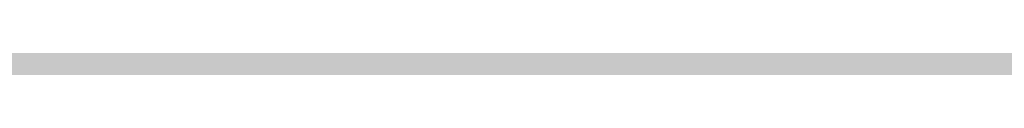
# Model space of a CAD drawing. Units: millimetres. Extents: x 0 to 2267, y 0 to 1823.
# Tile 79 of 256: x 1600.369 to 1605.705, y 1227.196 to 1227.23. Entities that reach past the tile are written whole.
import ezdxf

# ---------------------------------------------------------------- set-up
doc = ezdxf.new("R2010")
doc.units = ezdxf.units.MM
doc.header["$MEASUREMENT"] = 0
doc.layers.add('M-HATC', color=252, linetype='Continuous', lineweight=18)

msp = doc.modelspace()

# ---------------------------------------------------------------- hatches: boundary and pattern name
at = {"layer": 'M-HATC'}
h = msp.add_hatch(color=256, dxfattribs=at)
h.dxf.hatch_style = 1
h.paths.add_polyline_path([(2055.771, 1603.062), (1381.0868, 1603.062), (1381.0868, 1598.062), (2055.771, 1598.062)])
h.paths.add_polyline_path([(2055.771, 1598.062), (1381.0868, 1598.062), (1381.0868, 1593.062), (2055.771, 1593.062)])
h.paths.add_polyline_path([(2051.3074, 1536.7609), (1385.5504, 1536.7609), (1385.5504, 1526.7609), (1387.5504, 1526.7609), (1388.5366, 1525.0528), (1385.3319, 1521.2335), (1385.3319, 1521.2226), (2050.2542, 1522.7491), (2048.3212, 1525.0528), (2049.3074, 1526.7609), (2051.3074, 1526.7609)])
edge = h.paths.add_edge_path()
edge.add_arc((1847.5345, 1379.1492), 135, 222.603061, 222.890851, ccw=False)
edge.add_line((1748.1663, 1287.7656), (1683.0921, 1287.7656))
edge.add_arc((1583.7239, 1379.1492), 135, 317.109149, 317.396939, ccw=False)
edge.add_arc((1678.9686, 1290.6707), 5, 222.8909, 317.1091, ccw=False)
edge.add_arc((1774.2133, 1379.1492), 135, 222.603061, 222.890851, ccw=False)
edge.add_line((1674.8451, 1287.7656), (1609.7709, 1287.7656))
edge.add_arc((1510.4027, 1379.1492), 135, 317.109149, 317.396939, ccw=False)
edge.add_arc((1605.6474, 1290.6707), 5, 222.8909, 317.1091, ccw=False)
edge.add_arc((1700.8921, 1379.1492), 135, 222.603061, 222.890851, ccw=False)
edge.add_line((1601.5239, 1287.7656), (1536.4497, 1287.7656))
edge.add_arc((1437.0815, 1379.1492), 135, 317.109149, 317.396939, ccw=False)
edge.add_arc((1532.3262, 1290.6707), 5, 222.8909, 317.1091, ccw=False)
edge.add_arc((1627.5709, 1379.1492), 135, 222.603061, 222.890851, ccw=False)
edge.add_line((1528.2027, 1287.7656), (1505.9289, 1287.7656))
edge.add_spline(control_points=[(1505.9289, 1287.7656), (1504.2622, 1287.7656), (1504.2622, 1282.7656), (1505.9289, 1282.7656)], knot_values=[0, 0, 0, 0, 5, 5, 5, 5], degree=3, periodic=0)
edge.add_line((1505.9289, 1282.7656), (1930.9289, 1282.7656))
edge.add_spline(control_points=[(1930.9289, 1282.7656), (1932.5956, 1282.7656), (1932.5956, 1287.7656), (1930.9289, 1287.7656)], knot_values=[0, 0, 0, 0, 5, 5, 5, 5], degree=3, periodic=0)
edge.add_line((1930.9289, 1287.7656), (1903.0557, 1287.7656))
edge.add_arc((1803.6875, 1379.1492), 135, 317.109149, 317.396939, ccw=False)
edge.add_arc((1898.9322, 1290.6707), 5, 222.8909, 317.1091, ccw=False)
edge.add_arc((1994.1769, 1379.1492), 135, 222.603061, 222.890851, ccw=False)
edge.add_line((1894.8087, 1287.7656), (1829.7345, 1287.7656))
edge.add_arc((1730.3663, 1379.1492), 135, 317.109149, 317.396939, ccw=False)
edge.add_arc((1825.611, 1290.6707), 5, 222.8909, 317.1091, ccw=False)
edge.add_arc((1920.8557, 1379.1492), 135, 222.603061, 222.890851, ccw=False)
edge.add_line((1821.4875, 1287.7656), (1756.4133, 1287.7656))
edge.add_arc((1657.0451, 1379.1492), 135, 317.109149, 317.396939, ccw=False)
edge.add_arc((1752.2898, 1290.6707), 5, 222.8909, 317.1091, ccw=False)
edge = h.paths.add_edge_path()
edge.add_spline(control_points=[(1843.4289, 1227.2475), (1845.0956, 1227.2475), (1845.0956, 1232.2475), (1843.4289, 1232.2475)], knot_values=[0, 0, 0, 0, 5, 5, 5, 5], degree=3, periodic=0)
edge.add_line((1843.4289, 1232.2475), (1593.4289, 1232.2475))
edge.add_spline(control_points=[(1593.4289, 1232.2475), (1591.7622, 1232.2475), (1591.7622, 1227.2475), (1593.4289, 1227.2475)], knot_values=[0, 0, 0, 0, 5, 5, 5, 5], degree=3, periodic=0)
edge.add_line((1593.4289, 1227.2475), (1843.4289, 1227.2475))
h.paths.add_polyline_path([(1905.9289, 1127.4171), (1530.9289, 1127.4171, 0.414214), (1520.9289, 1117.4171), (1530.9289, 1117.4171), (1915.9289, 1117.4171, 0.414214)])
edge = h.paths.add_edge_path()
edge.add_arc((1397.0858, 1498.4078), 12.7299, 90.78215, 190.87871, ccw=False)
edge.add_line((1396.912, 1511.1365), (1428.0097, 1511.3488))
edge.add_line((1428.0097, 1511.3488), (1433.0097, 1511.3488))
edge.add_line((1433.0097, 1511.3488), (1434.439, 1511.3488))
edge.add_arc((1419.474, 1498.0804), 20, 41.561, 74.08211)
edge.add_line((1424.9592, 1517.3135), (1399.9351, 1517.2561))
edge.add_spline(control_points=[(1399.9307, 1517.2561), (1399.884, 1517.2131), (1399.8328, 1517.1689), (1399.7774, 1517.1236)], knot_values=[11.567499, 11.567499, 11.567499, 11.567499, 11.814249, 11.814249, 11.814249, 11.814249], degree=3, periodic=0)
edge.add_spline(control_points=[(1399.6328, 1517.0099), (1399.5831, 1516.9721), (1399.5307, 1516.9338), (1399.4759, 1516.8947)], knot_values=[11.167718, 11.167718, 11.167718, 11.167718, 11.365188, 11.365188, 11.365188, 11.365188], degree=3, periodic=0)
edge.add_spline(control_points=[(1399.3398, 1516.8001), (1399.1514, 1516.6719), (1398.9384, 1516.5377), (1398.704, 1516.3994)], knot_values=[10.376405, 10.376405, 10.376405, 10.376405, 11.00994, 11.00994, 11.00994, 11.00994], degree=3, periodic=0)
edge.add_spline(control_points=[(1398.6572, 1516.3719), (1398.5789, 1516.326), (1398.4983, 1516.2797), (1398.4155, 1516.2331)], knot_values=[10.125175, 10.125175, 10.125175, 10.125175, 10.334406, 10.334406, 10.334406, 10.334406], degree=3, periodic=0)
edge.add_spline(control_points=[(1398.2642, 1516.1487), (1398.196, 1516.1111), (1398.1263, 1516.0732), (1398.0555, 1516.0351)], knot_values=[9.832246, 9.832246, 9.832246, 9.832246, 9.999658, 9.999658, 9.999658, 9.999658], degree=3, periodic=0)
edge.add_spline(control_points=[(1397.9987, 1516.0048), (1397.7312, 1515.8621), (1397.446, 1515.7171), (1397.1466, 1515.5714)], knot_values=[9.161808, 9.161808, 9.161808, 9.161808, 9.787769, 9.787769, 9.787769, 9.787769], degree=3, periodic=0)
edge.add_spline(control_points=[(1397.1466, 1515.5714), (1396.8418, 1515.423), (1396.5222, 1515.274), (1396.1914, 1515.1262)], knot_values=[8.524455, 8.524455, 8.524455, 8.524455, 9.161808, 9.161808, 9.161808, 9.161808], degree=3, periodic=0)
edge.add_spline(control_points=[(1396.0777, 1515.0756), (1395.9854, 1515.0348), (1395.8922, 1514.994), (1395.7983, 1514.9534)], knot_values=[8.275193, 8.275193, 8.275193, 8.275193, 8.451726, 8.451726, 8.451726, 8.451726], degree=3, periodic=0)
edge.add_spline(control_points=[(1395.6018, 1514.8691), (1395.4997, 1514.8257), (1395.3968, 1514.7824), (1395.2932, 1514.7394)], knot_values=[7.962917, 7.962917, 7.962917, 7.962917, 8.152764, 8.152764, 8.152764, 8.152764], degree=3, periodic=0)
edge.add_spline(control_points=[(1395.2116, 1514.7057), (1394.8278, 1514.5475), (1394.4345, 1514.3929), (1394.0364, 1514.2442)], knot_values=[7.21254, 7.21254, 7.21254, 7.21254, 7.913148, 7.913148, 7.913148, 7.913148], degree=3, periodic=0)
edge.add_spline(control_points=[(1394.0364, 1514.2442), (1393.7076, 1514.1214), (1393.3754, 1514.0027), (1393.0427, 1513.8895)], knot_values=[6.633733, 6.633733, 6.633733, 6.633733, 7.21254, 7.21254, 7.21254, 7.21254], degree=3, periodic=0)
edge.add_spline(control_points=[(1392.8214, 1513.815), (1392.7198, 1513.7812), (1392.6181, 1513.7479), (1392.5166, 1513.7152)], knot_values=[6.328796, 6.328796, 6.328796, 6.328796, 6.505493, 6.505493, 6.505493, 6.505493], degree=3, periodic=0)
edge.add_spline(control_points=[(1392.5166, 1513.7152), (1392.3187, 1513.6515), (1392.1212, 1513.59), (1391.9244, 1513.531)], knot_values=[5.984605, 5.984605, 5.984605, 5.984605, 6.328796, 6.328796, 6.328796, 6.328796], degree=3, periodic=0)
edge.add_spline(control_points=[(1391.7915, 1513.4915), (1391.3122, 1513.3501), (1390.8384, 1513.2239), (1390.3784, 1513.1171)], knot_values=[5.066697, 5.066697, 5.066697, 5.066697, 5.907055, 5.907055, 5.907055, 5.907055], degree=3, periodic=0)
edge.add_spline(control_points=[(1390.3784, 1513.1171), (1390.1797, 1513.071), (1389.9836, 1513.0284), (1389.7907, 1512.9899)], knot_values=[4.70367, 4.70367, 4.70367, 4.70367, 5.066695, 5.066695, 5.066695, 5.066695], degree=3, periodic=0)
edge.add_spline(control_points=[(1389.422, 1512.9204), (1389.2459, 1512.8892), (1389.0729, 1512.8617), (1388.9036, 1512.8381)], knot_values=[4.130571, 4.130571, 4.130571, 4.130571, 4.469816, 4.469816, 4.469816, 4.469816], degree=3, periodic=0)
edge.add_spline(control_points=[(1388.9036, 1512.8381), (1388.591, 1512.7946), (1388.2911, 1512.7644), (1388.0071, 1512.7494)], knot_values=[3.504031, 3.504031, 3.504031, 3.504031, 4.130571, 4.130571, 4.130571, 4.130571], degree=3, periodic=0)
edge.add_spline(control_points=[(1387.9356, 1512.7459), (1387.8538, 1512.7423), (1387.7733, 1512.74), (1387.6944, 1512.739)], knot_values=[3.268866, 3.268866, 3.268866, 3.268866, 3.451164, 3.451164, 3.451164, 3.451164], degree=3, periodic=0)
edge.add_spline(control_points=[(1387.3351, 1512.7443), (1387.2076, 1512.7499), (1387.0847, 1512.7597), (1386.967, 1512.7739)], knot_values=[2.670686, 2.670686, 2.670686, 2.670686, 2.984, 2.984, 2.984, 2.984], degree=3, periodic=0)
edge.add_spline(control_points=[(1386.8327, 1512.7922), (1386.8209, 1512.7941), (1386.8092, 1512.7959), (1386.7975, 1512.7979)], knot_values=[2.516981, 2.516981, 2.516981, 2.516981, 2.549528, 2.549528, 2.549528, 2.549528], degree=3, periodic=0)
edge.add_spline(control_points=[(1386.4526, 1512.8735), (1386.4257, 1512.881), (1386.3993, 1512.889), (1386.3733, 1512.8972)], knot_values=[2.095869, 2.095869, 2.095869, 2.095869, 2.17941, 2.17941, 2.17941, 2.17941], degree=3, periodic=0)
edge.add_spline(control_points=[(1386.0691, 1513.0189), (1386.0634, 1513.0217), (1386.0577, 1513.0246), (1386.052, 1513.0275)], knot_values=[1.72453, 1.72453, 1.72453, 1.72453, 1.745933, 1.745933, 1.745933, 1.745933], degree=3, periodic=0)
edge.add_arc((1399.474, 1498.0804), 20, 131.82432, 180)
edge.add_arc((1630.3336, 1505.5484), 250.9708, 181.705176, 236.427975)
edge.add_arc((1605.3399, 1483.3044), 218.7822, 238.660829, 243.34961)
edge.add_arc((1647.0911, 1510.3592), 262.8986, 183.129836, 237.853442, ccw=False)
h.paths.add_polyline_path([(1406.5369, 1391.9644, 0.149382), (1491.5506, 1296.4418, -0.129517)], flags=17)
edge = h.paths.add_edge_path()
edge.add_arc((2037.3838, 1498.0804), 20, 0, 48.26587)
edge.add_spline(control_points=[(2050.6973, 1513.0052), (2050.6512, 1512.9847), (2050.6034, 1512.9655), (2050.5539, 1512.9477)], knot_values=[1.835652, 1.835652, 1.835652, 1.835652, 2.000781, 2.000781, 2.000781, 2.000781], degree=3, periodic=0)
edge.add_spline(control_points=[(2050.4616, 1512.9166), (2050.479, 1512.9221), (2050.4963, 1512.9277), (2050.5133, 1512.9335)], knot_values=[2.045477, 2.045477, 2.045477, 2.045477, 2.101389, 2.101389, 2.101389, 2.101389], degree=3, periodic=0)
edge.add_spline(control_points=[(2050.129, 1512.8342), (2050.1984, 1512.8473), (2050.2657, 1512.8623), (2050.3308, 1512.8792)], knot_values=[2.237629, 2.237629, 2.237629, 2.237629, 2.435841, 2.435841, 2.435841, 2.435841], degree=3, periodic=0)
edge.add_spline(control_points=[(2050.0946, 1512.8278), (2050.1061, 1512.8299), (2050.1176, 1512.832), (2050.129, 1512.8342)], knot_values=[2.435841, 2.435841, 2.435841, 2.435841, 2.468321, 2.468321, 2.468321, 2.468321], degree=3, periodic=0)
edge.add_spline(control_points=[(2049.7843, 1512.7851), (2049.8552, 1512.7922), (2049.9243, 1512.8008), (2049.9917, 1512.8109)], knot_values=[2.563852, 2.563852, 2.563852, 2.563852, 2.748541, 2.748541, 2.748541, 2.748541], degree=3, periodic=0)
edge.add_spline(control_points=[(2049.4052, 1512.7617), (2049.5364, 1512.7653), (2049.6629, 1512.773), (2049.7843, 1512.7851)], knot_values=[2.748541, 2.748541, 2.748541, 2.748541, 3.064882, 3.064882, 3.064882, 3.064882], degree=3, periodic=0)
edge.add_spline(control_points=[(2049.1698, 1512.7597), (2049.2336, 1512.7591), (2049.2965, 1512.7594), (2049.3584, 1512.7606)], knot_values=[3.102309, 3.102309, 3.102309, 3.102309, 3.2503, 3.2503, 3.2503, 3.2503], degree=3, periodic=0)
edge.add_spline(control_points=[(2048.8573, 1512.7691), (2048.9638, 1512.7638), (2049.068, 1512.7606), (2049.1698, 1512.7597)], knot_values=[3.2503, 3.2503, 3.2503, 3.2503, 3.486069, 3.486069, 3.486069, 3.486069], degree=3, periodic=0)
edge.add_spline(control_points=[(2048.6924, 1512.7789), (2048.3729, 1512.8009), (2048.0345, 1512.8411), (2047.6817, 1512.897)], knot_values=[3.606429, 3.606429, 3.606429, 3.606429, 4.2989, 4.2989, 4.2989, 4.2989], degree=3, periodic=0)
edge.add_spline(control_points=[(2047.6817, 1512.897), (2047.5458, 1512.9185), (2047.4077, 1512.9424), (2047.2678, 1512.9685)], knot_values=[4.2989, 4.2989, 4.2989, 4.2989, 4.565769, 4.565769, 4.565769, 4.565769], degree=3, periodic=0)
edge.add_spline(control_points=[(2047.2678, 1512.9685), (2047.1449, 1512.9914), (2047.0207, 1513.016), (2046.8951, 1513.0422)], knot_values=[4.565769, 4.565769, 4.565769, 4.565769, 4.799971, 4.799971, 4.799971, 4.799971], degree=3, periodic=0)
edge.add_spline(control_points=[(2046.8951, 1513.0422), (2046.5286, 1513.1188), (2046.1513, 1513.209), (2045.7676, 1513.3107)], knot_values=[4.799971, 4.799971, 4.799971, 4.799971, 5.483718, 5.483718, 5.483718, 5.483718], degree=3, periodic=0)
edge.add_spline(control_points=[(2045.7676, 1513.3107), (2045.3724, 1513.4154), (2044.9704, 1513.5322), (2044.5662, 1513.6588)], knot_values=[5.483718, 5.483718, 5.483718, 5.483718, 6.187866, 6.187866, 6.187866, 6.187866], degree=3, periodic=0)
edge.add_spline(control_points=[(2044.5662, 1513.6588), (2044.4149, 1513.7061), (2044.2633, 1513.7549), (2044.1116, 1513.8048)], knot_values=[6.187866, 6.187866, 6.187866, 6.187866, 6.451551, 6.451551, 6.451551, 6.451551], degree=3, periodic=0)
edge.add_spline(control_points=[(2044.1116, 1513.8048), (2043.9967, 1513.8427), (2043.8817, 1513.8813), (2043.7668, 1513.9205)], knot_values=[6.451551, 6.451551, 6.451551, 6.451551, 6.651434, 6.651434, 6.651434, 6.651434], degree=3, periodic=0)
edge.add_spline(control_points=[(2043.7668, 1513.9205), (2043.3716, 1514.0554), (2042.9774, 1514.1979), (2042.5886, 1514.3458)], knot_values=[6.651434, 6.651434, 6.651434, 6.651434, 7.338879, 7.338879, 7.338879, 7.338879], degree=3, periodic=0)
edge.add_spline(control_points=[(2042.5886, 1514.3458), (2042.1643, 1514.5071), (2041.7465, 1514.6749), (2041.3409, 1514.846)], knot_values=[7.338879, 7.338879, 7.338879, 7.338879, 8.089209, 8.089209, 8.089209, 8.089209], degree=3, periodic=0)
edge.add_spline(control_points=[(2041.3409, 1514.846), (2041.1028, 1514.9465), (2040.869, 1515.0481), (2040.6405, 1515.1502)], knot_values=[8.089209, 8.089209, 8.089209, 8.089209, 8.529587, 8.529587, 8.529587, 8.529587], degree=3, periodic=0)
edge.add_spline(control_points=[(2040.51, 1515.2089), (2040.0824, 1515.4022), (2039.6747, 1515.5971), (2039.295, 1515.7894)], knot_values=[8.613818, 8.613818, 8.613818, 8.613818, 9.44571, 9.44571, 9.44571, 9.44571], degree=3, periodic=0)
edge.add_spline(control_points=[(2039.295, 1515.7894), (2039.0618, 1515.9075), (2038.8391, 1516.0246), (2038.6288, 1516.1398)], knot_values=[9.44571, 9.44571, 9.44571, 9.44571, 9.956404, 9.956404, 9.956404, 9.956404], degree=3, periodic=0)
edge.add_spline(control_points=[(2038.6288, 1516.1398), (2038.5187, 1516.2001), (2038.4121, 1516.2598), (2038.309, 1516.3189)], knot_values=[9.956404, 9.956404, 9.956404, 9.956404, 10.223542, 10.223542, 10.223542, 10.223542], degree=3, periodic=0)
edge.add_spline(control_points=[(2038.309, 1516.3189), (2038.2138, 1516.3735), (2038.1216, 1516.4276), (2038.0328, 1516.481)], knot_values=[10.223542, 10.223542, 10.223542, 10.223542, 10.47051, 10.47051, 10.47051, 10.47051], degree=3, periodic=0)
edge.add_spline(control_points=[(2038.0328, 1516.481), (2037.7855, 1516.6296), (2037.5639, 1516.773), (2037.3722, 1516.909)], knot_values=[10.47051, 10.47051, 10.47051, 10.47051, 11.15767, 11.15767, 11.15767, 11.15767], degree=3, periodic=0)
edge.add_spline(control_points=[(2037.3722, 1516.909), (2037.2789, 1516.9752), (2037.1927, 1517.0396), (2037.1142, 1517.102)], knot_values=[11.15767, 11.15767, 11.15767, 11.15767, 11.49227, 11.49227, 11.49227, 11.49227], degree=3, periodic=0)
edge.add_spline(control_points=[(2036.8564, 1517.3259), (2036.9148, 1517.2692), (2036.9814, 1517.2103), (2037.0557, 1517.1492)], knot_values=[11.577341, 11.577341, 11.577341, 11.577341, 11.91035, 11.91035, 11.91035, 11.91035], degree=3, periodic=0)
edge.add_spline(control_points=[(2036.8074, 1517.3748), (2036.823, 1517.3587), (2036.8393, 1517.3424), (2036.8564, 1517.3259)], knot_values=[11.91035, 11.91035, 11.91035, 11.91035, 12.007402, 12.007402, 12.007402, 12.007402], degree=3, periodic=0)
edge.add_spline(control_points=[(2036.7017, 1517.494), (2036.7104, 1517.483), (2036.7196, 1517.4719), (2036.7291, 1517.4606)], knot_values=[12.184155, 12.184155, 12.184155, 12.184155, 12.255409, 12.255409, 12.255409, 12.255409], degree=3, periodic=0)
edge.add_spline(control_points=[(2036.6159, 1517.6205), (2036.62, 1517.613), (2036.6243, 1517.6055), (2036.6289, 1517.5979)], knot_values=[12.487913, 12.487913, 12.487913, 12.487913, 12.541035, 12.541035, 12.541035, 12.541035], degree=3, periodic=0)
edge.add_spline(control_points=[(2036.5635, 1517.786), (2036.5637, 1517.7794), (2036.5642, 1517.7726), (2036.565, 1517.7658)], knot_values=[12.911761, 12.911761, 12.911761, 12.911761, 12.968286, 12.968286, 12.968286, 12.968286], degree=3, periodic=0)
edge.add_spline(control_points=[(2036.6166, 1517.9304), (2036.6125, 1517.9259), (2036.6086, 1517.9212), (2036.6049, 1517.9165)], knot_values=[13.382527, 13.382527, 13.382527, 13.382527, 13.433791, 13.433791, 13.433791, 13.433791], degree=3, periodic=0)
edge.add_spline(control_points=[(2036.749, 1518.017), (2036.7361, 1518.0116), (2036.7239, 1518.006), (2036.7124, 1518.0002)], knot_values=[13.726299, 13.726299, 13.726299, 13.726299, 13.809928, 13.809928, 13.809928, 13.809928], degree=3, periodic=0)
edge.add_spline(control_points=[(2036.8604, 1518.0528), (2036.8386, 1518.0474), (2036.8181, 1518.0416), (2036.7988, 1518.0353)], knot_values=[13.910887, 13.910887, 13.910887, 13.910887, 14.02153, 14.02153, 14.02153, 14.02153], degree=3, periodic=0)
edge.add_line((2036.9639, 1518.0804), (2032.3838, 1518.0804))
edge.add_line((2032.3838, 1518.0804), (2027.3838, 1518.0804))
edge.add_line((2027.3838, 1518.0804), (2022.3838, 1518.0804))
edge.add_line((2022.3838, 1518.0804), (2017.3838, 1518.0804))
edge.add_arc((2017.3838, 1498.0804), 20, 90, 138.439)
edge.add_line((2002.4188, 1511.3488), (2003.8481, 1511.3488))
edge.add_line((2003.8481, 1511.3488), (2008.8481, 1511.3488))
edge.add_line((2008.8481, 1511.3488), (2039.772, 1511.1377))
edge.add_arc((2039.772, 1498.4078), 12.7299, -10.87871, 90, ccw=False)
edge.add_arc((1789.7668, 1510.3592), 262.8986, 302.146558, 356.870164, ccw=False)
edge.add_arc((1831.5179, 1483.3044), 218.7822, 296.65039, 301.339171)
edge.add_arc((1806.5242, 1505.5484), 250.9708, 303.572025, 358.294824)
h.paths.add_polyline_path([(2030.321, 1391.9644, -0.129517), (1945.3072, 1296.4418, 0.149382)], flags=17)
edge = h.paths.add_edge_path()
edge.add_spline(control_points=[(2037.2464, 1518.0821), (2037.2898, 1518.081), (2037.3355, 1518.0804), (2037.3838, 1518.0804)], knot_values=[0.000012, 0.000012, 0.000012, 0.000012, 0.144754, 0.144754, 0.144754, 0.144754], degree=3, periodic=0)
edge.add_line((2037.3357, 1518.0804), (2037.0096, 1518.0804))
edge.add_spline(control_points=[(2037.0096, 1518.0804), (2036.9822, 1518.0768), (2036.956, 1518.0727), (2036.9312, 1518.0681)], knot_values=[14.13465, 14.13465, 14.13465, 14.13465, 14.247197, 14.247197, 14.247197, 14.247197], degree=3, periodic=0)
edge.add_spline(control_points=[(2036.9312, 1518.0681), (2036.9276, 1518.0674), (2036.9241, 1518.0667), (2036.9205, 1518.0661)], knot_values=[14.118315, 14.118315, 14.118315, 14.118315, 14.13465, 14.13465, 14.13465, 14.13465], degree=3, periodic=0)
edge.add_spline(control_points=[(2036.9205, 1518.0661), (2036.9118, 1518.0644), (2036.9032, 1518.0626), (2036.8948, 1518.0608)], knot_values=[14.078086, 14.078086, 14.078086, 14.078086, 14.118315, 14.118315, 14.118315, 14.118315], degree=3, periodic=0)
edge.add_spline(control_points=[(2036.8948, 1518.0608), (2036.883, 1518.0583), (2036.8716, 1518.0556), (2036.8604, 1518.0528)], knot_values=[14.02153, 14.02153, 14.02153, 14.02153, 14.078086, 14.078086, 14.078086, 14.078086], degree=3, periodic=0)
edge.add_spline(control_points=[(2036.8604, 1518.0528), (2036.8386, 1518.0474), (2036.8181, 1518.0416), (2036.7988, 1518.0353)], knot_values=[13.910887, 13.910887, 13.910887, 13.910887, 14.02153, 14.02153, 14.02153, 14.02153], degree=3, periodic=0)
edge.add_spline(control_points=[(2036.7988, 1518.0353), (2036.7981, 1518.035), (2036.7974, 1518.0348), (2036.7967, 1518.0346)], knot_values=[13.906906, 13.906906, 13.906906, 13.906906, 13.910887, 13.910887, 13.910887, 13.910887], degree=3, periodic=0)
edge.add_spline(control_points=[(2036.7967, 1518.0346), (2036.7882, 1518.0318), (2036.7799, 1518.0289), (2036.7719, 1518.0259)], knot_values=[13.857826, 13.857826, 13.857826, 13.857826, 13.906906, 13.906906, 13.906906, 13.906906], degree=3, periodic=0)
edge.add_spline(control_points=[(2036.7719, 1518.0259), (2036.764, 1518.023), (2036.7564, 1518.02), (2036.749, 1518.017)], knot_values=[13.809928, 13.809928, 13.809928, 13.809928, 13.857826, 13.857826, 13.857826, 13.857826], degree=3, periodic=0)
edge.add_spline(control_points=[(2036.749, 1518.017), (2036.7361, 1518.0116), (2036.7239, 1518.006), (2036.7124, 1518.0002)], knot_values=[13.726299, 13.726299, 13.726299, 13.726299, 13.809928, 13.809928, 13.809928, 13.809928], degree=3, periodic=0)
edge.add_spline(control_points=[(2036.7124, 1518.0002), (2036.7121, 1518), (2036.7118, 1517.9999), (2036.7115, 1517.9997)], knot_values=[13.723993, 13.723993, 13.723993, 13.723993, 13.726299, 13.726299, 13.726299, 13.726299], degree=3, periodic=0)
edge.add_spline(control_points=[(2036.7115, 1517.9997), (2036.7063, 1517.9971), (2036.7013, 1517.9944), (2036.6965, 1517.9917)], knot_values=[13.686536, 13.686536, 13.686536, 13.686536, 13.723993, 13.723993, 13.723993, 13.723993], degree=3, periodic=0)
edge.add_spline(control_points=[(2036.6965, 1517.9917), (2036.6919, 1517.9891), (2036.6874, 1517.9865), (2036.6831, 1517.9839)], knot_values=[13.651251, 13.651251, 13.651251, 13.651251, 13.686536, 13.686536, 13.686536, 13.686536], degree=3, periodic=0)
edge.add_spline(control_points=[(2036.6831, 1517.9839), (2036.6764, 1517.9798), (2036.67, 1517.9757), (2036.6639, 1517.9714)], knot_values=[13.596804, 13.596804, 13.596804, 13.596804, 13.651251, 13.651251, 13.651251, 13.651251], degree=3, periodic=0)
edge.add_spline(control_points=[(2036.6639, 1517.9714), (2036.6636, 1517.9712), (2036.6633, 1517.9709), (2036.6629, 1517.9707)], knot_values=[13.593956, 13.593956, 13.593956, 13.593956, 13.596804, 13.596804, 13.596804, 13.596804], degree=3, periodic=0)
edge.add_spline(control_points=[(2036.6629, 1517.9707), (2036.6603, 1517.9689), (2036.6577, 1517.967), (2036.6552, 1517.9651)], knot_values=[13.570322, 13.570322, 13.570322, 13.570322, 13.593956, 13.593956, 13.593956, 13.593956], degree=3, periodic=0)
edge.add_spline(control_points=[(2036.6552, 1517.9651), (2036.6525, 1517.9631), (2036.6499, 1517.9611), (2036.6474, 1517.9591)], knot_values=[13.545477, 13.545477, 13.545477, 13.545477, 13.570322, 13.570322, 13.570322, 13.570322], degree=3, periodic=0)
edge.add_spline(control_points=[(2036.6474, 1517.9591), (2036.6472, 1517.9589), (2036.6471, 1517.9588), (2036.6469, 1517.9587)], knot_values=[13.543931, 13.543931, 13.543931, 13.543931, 13.545477, 13.545477, 13.545477, 13.545477], degree=3, periodic=0)
edge.add_spline(control_points=[(2036.6469, 1517.9587), (2036.6412, 1517.9541), (2036.6358, 1517.9494), (2036.6307, 1517.9447)], knot_values=[13.488237, 13.488237, 13.488237, 13.488237, 13.543931, 13.543931, 13.543931, 13.543931], degree=3, periodic=0)
edge.add_spline(control_points=[(2036.6307, 1517.9447), (2036.6282, 1517.9423), (2036.6257, 1517.9399), (2036.6233, 1517.9374)], knot_values=[13.460307, 13.460307, 13.460307, 13.460307, 13.488237, 13.488237, 13.488237, 13.488237], degree=3, periodic=0)
edge.add_spline(control_points=[(2036.6233, 1517.9374), (2036.6215, 1517.9356), (2036.6198, 1517.9338), (2036.6181, 1517.932)], knot_values=[13.439712, 13.439712, 13.439712, 13.439712, 13.460307, 13.460307, 13.460307, 13.460307], degree=3, periodic=0)
edge.add_spline(control_points=[(2036.6181, 1517.932), (2036.6176, 1517.9315), (2036.6171, 1517.9309), (2036.6166, 1517.9304)], knot_values=[13.433791, 13.433791, 13.433791, 13.433791, 13.439712, 13.439712, 13.439712, 13.439712], degree=3, periodic=0)
edge.add_spline(control_points=[(2036.6166, 1517.9304), (2036.6125, 1517.9259), (2036.6086, 1517.9212), (2036.6049, 1517.9165)], knot_values=[13.382527, 13.382527, 13.382527, 13.382527, 13.433791, 13.433791, 13.433791, 13.433791], degree=3, periodic=0)
edge.add_spline(control_points=[(2036.6049, 1517.9165), (2036.6026, 1517.9135), (2036.6004, 1517.9104), (2036.5982, 1517.9074)], knot_values=[13.350017, 13.350017, 13.350017, 13.350017, 13.382527, 13.382527, 13.382527, 13.382527], degree=3, periodic=0)
edge.add_spline(control_points=[(2036.5982, 1517.9074), (2036.5972, 1517.9059), (2036.5962, 1517.9043), (2036.5952, 1517.9028)], knot_values=[13.333922, 13.333922, 13.333922, 13.333922, 13.350017, 13.350017, 13.350017, 13.350017], degree=3, periodic=0)
edge.add_spline(control_points=[(2036.5952, 1517.9028), (2036.5945, 1517.9018), (2036.5939, 1517.9009), (2036.5933, 1517.8999)], knot_values=[13.323828, 13.323828, 13.323828, 13.323828, 13.333922, 13.333922, 13.333922, 13.333922], degree=3, periodic=0)
edge.add_spline(control_points=[(2036.5933, 1517.8999), (2036.5905, 1517.8955), (2036.5879, 1517.8909), (2036.5855, 1517.8864)], knot_values=[13.277545, 13.277545, 13.277545, 13.277545, 13.323828, 13.323828, 13.323828, 13.323828], degree=3, periodic=0)
edge.add_spline(control_points=[(2036.5855, 1517.8864), (2036.5836, 1517.8827), (2036.5817, 1517.8789), (2036.5801, 1517.8751)], knot_values=[13.240119, 13.240119, 13.240119, 13.240119, 13.277545, 13.277545, 13.277545, 13.277545], degree=3, periodic=0)
edge.add_spline(control_points=[(2036.5801, 1517.8751), (2036.5795, 1517.8739), (2036.579, 1517.8727), (2036.5785, 1517.8715)], knot_values=[13.228211, 13.228211, 13.228211, 13.228211, 13.240119, 13.240119, 13.240119, 13.240119], degree=3, periodic=0)
edge.add_spline(control_points=[(2036.5785, 1517.8715), (2036.578, 1517.8702), (2036.5774, 1517.869), (2036.5769, 1517.8677)], knot_values=[13.215717, 13.215717, 13.215717, 13.215717, 13.228211, 13.228211, 13.228211, 13.228211], degree=3, periodic=0)
edge.add_spline(control_points=[(2036.5769, 1517.8677), (2036.5755, 1517.864), (2036.5741, 1517.8603), (2036.5729, 1517.8565)], knot_values=[13.179847, 13.179847, 13.179847, 13.179847, 13.215717, 13.215717, 13.215717, 13.215717], degree=3, periodic=0)
edge.add_spline(control_points=[(2036.5729, 1517.8565), (2036.5713, 1517.8515), (2036.5699, 1517.8464), (2036.5687, 1517.8413)], knot_values=[13.132017, 13.132017, 13.132017, 13.132017, 13.179847, 13.179847, 13.179847, 13.179847], degree=3, periodic=0)
edge.add_spline(control_points=[(2036.5687, 1517.8413), (2036.5684, 1517.8402), (2036.5682, 1517.8392), (2036.568, 1517.8382)], knot_values=[13.122482, 13.122482, 13.122482, 13.122482, 13.132017, 13.132017, 13.132017, 13.132017], degree=3, periodic=0)
edge.add_spline(control_points=[(2036.568, 1517.8382), (2036.5676, 1517.8363), (2036.5672, 1517.8345), (2036.5669, 1517.8327)], knot_values=[13.105592, 13.105592, 13.105592, 13.105592, 13.122482, 13.122482, 13.122482, 13.122482], degree=3, periodic=0)
edge.add_spline(control_points=[(2036.5669, 1517.8327), (2036.5662, 1517.8292), (2036.5657, 1517.8257), (2036.5652, 1517.8222)], knot_values=[13.074063, 13.074063, 13.074063, 13.074063, 13.105592, 13.105592, 13.105592, 13.105592], degree=3, periodic=0)
edge.add_spline(control_points=[(2036.5652, 1517.8222), (2036.5652, 1517.8222), (2036.5652, 1517.8222), (2036.5652, 1517.8222)], knot_values=[13.074043, 13.074043, 13.074043, 13.074043, 13.074063, 13.074063, 13.074063, 13.074063], degree=3, periodic=0)
edge.add_spline(control_points=[(2036.5652, 1517.8222), (2036.5644, 1517.8164), (2036.5639, 1517.8106), (2036.5636, 1517.8046)], knot_values=[13.021884, 13.021884, 13.021884, 13.021884, 13.074043, 13.074043, 13.074043, 13.074043], degree=3, periodic=0)
edge.add_spline(control_points=[(2036.5636, 1517.8046), (2036.5636, 1517.804), (2036.5636, 1517.8034), (2036.5635, 1517.8028)], knot_values=[13.01674, 13.01674, 13.01674, 13.01674, 13.021884, 13.021884, 13.021884, 13.021884], degree=3, periodic=0)
edge.add_spline(control_points=[(2036.5635, 1517.8028), (2036.5634, 1517.8005), (2036.5634, 1517.7982), (2036.5634, 1517.7958)], knot_values=[12.996438, 12.996438, 12.996438, 12.996438, 13.01674, 13.01674, 13.01674, 13.01674], degree=3, periodic=0)
edge.add_spline(control_points=[(2036.5634, 1517.7958), (2036.5633, 1517.7926), (2036.5634, 1517.7893), (2036.5635, 1517.786)], knot_values=[12.968286, 12.968286, 12.968286, 12.968286, 12.996438, 12.996438, 12.996438, 12.996438], degree=3, periodic=0)
edge.add_spline(control_points=[(2036.5635, 1517.786), (2036.5637, 1517.7794), (2036.5642, 1517.7726), (2036.565, 1517.7658)], knot_values=[12.911761, 12.911761, 12.911761, 12.911761, 12.968286, 12.968286, 12.968286, 12.968286], degree=3, periodic=0)
edge.add_spline(control_points=[(2036.565, 1517.7658), (2036.565, 1517.7657), (2036.565, 1517.7656), (2036.565, 1517.7656)], knot_values=[12.911017, 12.911017, 12.911017, 12.911017, 12.911761, 12.911761, 12.911761, 12.911761], degree=3, periodic=0)
edge.add_spline(control_points=[(2036.565, 1517.7656), (2036.5654, 1517.7625), (2036.5658, 1517.7593), (2036.5663, 1517.7562)], knot_values=[12.88528, 12.88528, 12.88528, 12.88528, 12.911017, 12.911017, 12.911017, 12.911017], degree=3, periodic=0)
edge.add_spline(control_points=[(2036.5663, 1517.7562), (2036.5667, 1517.7534), (2036.5672, 1517.7506), (2036.5677, 1517.7478)], knot_values=[12.862519, 12.862519, 12.862519, 12.862519, 12.88528, 12.88528, 12.88528, 12.88528], degree=3, periodic=0)
edge.add_spline(control_points=[(2036.5677, 1517.7478), (2036.5678, 1517.7474), (2036.5679, 1517.7469), (2036.568, 1517.7465)], knot_values=[12.858885, 12.858885, 12.858885, 12.858885, 12.862519, 12.862519, 12.862519, 12.862519], degree=3, periodic=0)
edge.add_spline(control_points=[(2036.568, 1517.7465), (2036.5692, 1517.7399), (2036.5707, 1517.7332), (2036.5724, 1517.7264)], knot_values=[12.8053, 12.8053, 12.8053, 12.8053, 12.858885, 12.858885, 12.858885, 12.858885], degree=3, periodic=0)
edge.add_spline(control_points=[(2036.5724, 1517.7264), (2036.5734, 1517.7226), (2036.5745, 1517.7187), (2036.5756, 1517.7149)], knot_values=[12.775176, 12.775176, 12.775176, 12.775176, 12.8053, 12.8053, 12.8053, 12.8053], degree=3, periodic=0)
edge.add_spline(control_points=[(2036.5756, 1517.7149), (2036.5763, 1517.7125), (2036.577, 1517.7102), (2036.5778, 1517.7078)], knot_values=[12.756759, 12.756759, 12.756759, 12.756759, 12.775176, 12.775176, 12.775176, 12.775176], degree=3, periodic=0)
edge.add_spline(control_points=[(2036.5778, 1517.7078), (2036.5781, 1517.7067), (2036.5784, 1517.7057), (2036.5787, 1517.7047)], knot_values=[12.748742, 12.748742, 12.748742, 12.748742, 12.756759, 12.756759, 12.756759, 12.756759], degree=3, periodic=0)
edge.add_spline(control_points=[(2036.5787, 1517.7047), (2036.5808, 1517.6983), (2036.5831, 1517.6919), (2036.5856, 1517.6854)], knot_values=[12.69959, 12.69959, 12.69959, 12.69959, 12.748742, 12.748742, 12.748742, 12.748742], degree=3, periodic=0)
edge.add_spline(control_points=[(2036.5856, 1517.6854), (2036.5876, 1517.68), (2036.5898, 1517.6746), (2036.5921, 1517.6692)], knot_values=[12.659038, 12.659038, 12.659038, 12.659038, 12.69959, 12.69959, 12.69959, 12.69959], degree=3, periodic=0)
edge.add_spline(control_points=[(2036.5921, 1517.6692), (2036.594, 1517.6648), (2036.5959, 1517.6605), (2036.5979, 1517.6561)], knot_values=[12.626806, 12.626806, 12.626806, 12.626806, 12.659038, 12.659038, 12.659038, 12.659038], degree=3, periodic=0)
edge.add_spline(control_points=[(2036.5979, 1517.6561), (2036.5984, 1517.6551), (2036.5989, 1517.6541), (2036.5993, 1517.6531)], knot_values=[12.619394, 12.619394, 12.619394, 12.619394, 12.626806, 12.626806, 12.626806, 12.626806], degree=3, periodic=0)
edge.add_spline(control_points=[(2036.5993, 1517.6531), (2036.6043, 1517.6424), (2036.6099, 1517.6315), (2036.6159, 1517.6205)], knot_values=[12.541039, 12.541039, 12.541039, 12.541039, 12.619394, 12.619394, 12.619394, 12.619394], degree=3, periodic=0)
edge.add_spline(control_points=[(2036.6159, 1517.6205), (2036.6159, 1517.6205), (2036.6159, 1517.6205), (2036.6159, 1517.6205)], knot_values=[12.541035, 12.541035, 12.541035, 12.541035, 12.541039, 12.541039, 12.541039, 12.541039], degree=3, periodic=0)
edge.add_spline(control_points=[(2036.6159, 1517.6205), (2036.62, 1517.613), (2036.6243, 1517.6055), (2036.6289, 1517.5979)], knot_values=[12.487913, 12.487913, 12.487913, 12.487913, 12.541035, 12.541035, 12.541035, 12.541035], degree=3, periodic=0)
edge.add_spline(control_points=[(2036.6289, 1517.5979), (2036.6326, 1517.5916), (2036.6365, 1517.5853), (2036.6406, 1517.5789)], knot_values=[12.443982, 12.443982, 12.443982, 12.443982, 12.487913, 12.487913, 12.487913, 12.487913], degree=3, periodic=0)
edge.add_spline(control_points=[(2036.6406, 1517.5789), (2036.6414, 1517.5776), (2036.6423, 1517.5763), (2036.6431, 1517.5749)], knot_values=[12.434996, 12.434996, 12.434996, 12.434996, 12.443982, 12.443982, 12.443982, 12.443982], degree=3, periodic=0)
edge.add_spline(control_points=[(2036.6431, 1517.5749), (2036.6531, 1517.5596), (2036.6639, 1517.5439), (2036.6756, 1517.528)], knot_values=[12.329647, 12.329647, 12.329647, 12.329647, 12.434996, 12.434996, 12.434996, 12.434996], degree=3, periodic=0)
edge.add_spline(control_points=[(2036.6756, 1517.528), (2036.6839, 1517.5168), (2036.6925, 1517.5055), (2036.7017, 1517.494)], knot_values=[12.255409, 12.255409, 12.255409, 12.255409, 12.329647, 12.329647, 12.329647, 12.329647], degree=3, periodic=0)
edge.add_spline(control_points=[(2036.7017, 1517.494), (2036.7104, 1517.483), (2036.7196, 1517.4719), (2036.7291, 1517.4606)], knot_values=[12.184155, 12.184155, 12.184155, 12.184155, 12.255409, 12.255409, 12.255409, 12.255409], degree=3, periodic=0)
edge.add_spline(control_points=[(2036.7291, 1517.4606), (2036.7436, 1517.4435), (2036.759, 1517.4262), (2036.7753, 1517.4085)], knot_values=[12.075961, 12.075961, 12.075961, 12.075961, 12.184155, 12.184155, 12.184155, 12.184155], degree=3, periodic=0)
edge.add_spline(control_points=[(2036.7753, 1517.4085), (2036.7763, 1517.4075), (2036.7773, 1517.4064), (2036.7783, 1517.4054)], knot_values=[12.069502, 12.069502, 12.069502, 12.069502, 12.075961, 12.075961, 12.075961, 12.075961], degree=3, periodic=0)
edge.add_spline(control_points=[(2036.7783, 1517.4054), (2036.7877, 1517.3953), (2036.7974, 1517.385), (2036.8074, 1517.3748)], knot_values=[12.007402, 12.007402, 12.007402, 12.007402, 12.069502, 12.069502, 12.069502, 12.069502], degree=3, periodic=0)
edge.add_spline(control_points=[(2036.8074, 1517.3748), (2036.823, 1517.3587), (2036.8393, 1517.3424), (2036.8564, 1517.3259)], knot_values=[11.91035, 11.91035, 11.91035, 11.91035, 12.007402, 12.007402, 12.007402, 12.007402], degree=3, periodic=0)
edge.add_spline(control_points=[(2036.8564, 1517.3259), (2036.9148, 1517.2692), (2036.9814, 1517.2103), (2037.0557, 1517.1492)], knot_values=[11.577341, 11.577341, 11.577341, 11.577341, 11.91035, 11.91035, 11.91035, 11.91035], degree=3, periodic=0)
edge.add_spline(control_points=[(2037.0557, 1517.1492), (2037.0747, 1517.1336), (2037.0942, 1517.1179), (2037.1142, 1517.102)], knot_values=[11.49227, 11.49227, 11.49227, 11.49227, 11.577341, 11.577341, 11.577341, 11.577341], degree=3, periodic=0)
edge.add_spline(control_points=[(2037.1142, 1517.102), (2037.1927, 1517.0396), (2037.2789, 1516.9752), (2037.3722, 1516.909)], knot_values=[11.15767, 11.15767, 11.15767, 11.15767, 11.49227, 11.49227, 11.49227, 11.49227], degree=3, periodic=0)
edge.add_spline(control_points=[(2037.3722, 1516.909), (2037.5639, 1516.773), (2037.7855, 1516.6296), (2038.0328, 1516.481)], knot_values=[10.47051, 10.47051, 10.47051, 10.47051, 11.15767, 11.15767, 11.15767, 11.15767], degree=3, periodic=0)
edge.add_spline(control_points=[(2038.0328, 1516.481), (2038.1216, 1516.4276), (2038.2138, 1516.3735), (2038.309, 1516.3189)], knot_values=[10.223542, 10.223542, 10.223542, 10.223542, 10.47051, 10.47051, 10.47051, 10.47051], degree=3, periodic=0)
edge.add_spline(control_points=[(2038.309, 1516.3189), (2038.4121, 1516.2598), (2038.5187, 1516.2001), (2038.6288, 1516.1398)], knot_values=[9.956404, 9.956404, 9.956404, 9.956404, 10.223542, 10.223542, 10.223542, 10.223542], degree=3, periodic=0)
edge.add_spline(control_points=[(2038.6288, 1516.1398), (2038.8391, 1516.0246), (2039.0618, 1515.9075), (2039.295, 1515.7894)], knot_values=[9.44571, 9.44571, 9.44571, 9.44571, 9.956404, 9.956404, 9.956404, 9.956404], degree=3, periodic=0)
edge.add_spline(control_points=[(2039.295, 1515.7894), (2039.6747, 1515.5971), (2040.0824, 1515.4022), (2040.51, 1515.2089)], knot_values=[8.613818, 8.613818, 8.613818, 8.613818, 9.44571, 9.44571, 9.44571, 9.44571], degree=3, periodic=0)
edge.add_spline(control_points=[(2040.51, 1515.2089), (2040.5533, 1515.1893), (2040.5968, 1515.1697), (2040.6405, 1515.1502)], knot_values=[8.529587, 8.529587, 8.529587, 8.529587, 8.613818, 8.613818, 8.613818, 8.613818], degree=3, periodic=0)
edge.add_spline(control_points=[(2040.6405, 1515.1502), (2040.869, 1515.0481), (2041.1028, 1514.9465), (2041.3409, 1514.846)], knot_values=[8.089209, 8.089209, 8.089209, 8.089209, 8.529587, 8.529587, 8.529587, 8.529587], degree=3, periodic=0)
edge.add_spline(control_points=[(2041.3409, 1514.846), (2041.7465, 1514.6749), (2042.1643, 1514.5071), (2042.5886, 1514.3458)], knot_values=[7.338879, 7.338879, 7.338879, 7.338879, 8.089209, 8.089209, 8.089209, 8.089209], degree=3, periodic=0)
edge.add_spline(control_points=[(2042.5886, 1514.3458), (2042.9774, 1514.1979), (2043.3716, 1514.0554), (2043.7668, 1513.9205)], knot_values=[6.651434, 6.651434, 6.651434, 6.651434, 7.338879, 7.338879, 7.338879, 7.338879], degree=3, periodic=0)
edge.add_spline(control_points=[(2043.7668, 1513.9205), (2043.8817, 1513.8813), (2043.9967, 1513.8427), (2044.1116, 1513.8048)], knot_values=[6.451551, 6.451551, 6.451551, 6.451551, 6.651434, 6.651434, 6.651434, 6.651434], degree=3, periodic=0)
edge.add_spline(control_points=[(2044.1116, 1513.8048), (2044.2633, 1513.7549), (2044.4149, 1513.7061), (2044.5662, 1513.6588)], knot_values=[6.187866, 6.187866, 6.187866, 6.187866, 6.451551, 6.451551, 6.451551, 6.451551], degree=3, periodic=0)
edge.add_spline(control_points=[(2044.5662, 1513.6588), (2044.9704, 1513.5322), (2045.3724, 1513.4154), (2045.7676, 1513.3107)], knot_values=[5.483718, 5.483718, 5.483718, 5.483718, 6.187866, 6.187866, 6.187866, 6.187866], degree=3, periodic=0)
edge.add_spline(control_points=[(2045.7676, 1513.3107), (2046.1513, 1513.209), (2046.5286, 1513.1188), (2046.8951, 1513.0422)], knot_values=[4.799971, 4.799971, 4.799971, 4.799971, 5.483718, 5.483718, 5.483718, 5.483718], degree=3, periodic=0)
edge.add_spline(control_points=[(2046.8951, 1513.0422), (2047.0207, 1513.016), (2047.1449, 1512.9914), (2047.2678, 1512.9685)], knot_values=[4.565769, 4.565769, 4.565769, 4.565769, 4.799971, 4.799971, 4.799971, 4.799971], degree=3, periodic=0)
edge.add_spline(control_points=[(2047.2678, 1512.9685), (2047.4077, 1512.9424), (2047.5458, 1512.9185), (2047.6817, 1512.897)], knot_values=[4.2989, 4.2989, 4.2989, 4.2989, 4.565769, 4.565769, 4.565769, 4.565769], degree=3, periodic=0)
edge.add_spline(control_points=[(2047.6817, 1512.897), (2048.0345, 1512.8411), (2048.3729, 1512.8009), (2048.6924, 1512.7789)], knot_values=[3.606429, 3.606429, 3.606429, 3.606429, 4.2989, 4.2989, 4.2989, 4.2989], degree=3, periodic=0)
edge.add_spline(control_points=[(2048.6924, 1512.7789), (2048.7479, 1512.7751), (2048.8029, 1512.7718), (2048.8573, 1512.7691)], knot_values=[3.486069, 3.486069, 3.486069, 3.486069, 3.606429, 3.606429, 3.606429, 3.606429], degree=3, periodic=0)
edge.add_spline(control_points=[(2048.8573, 1512.7691), (2048.9638, 1512.7638), (2049.068, 1512.7606), (2049.1698, 1512.7597)], knot_values=[3.2503, 3.2503, 3.2503, 3.2503, 3.486069, 3.486069, 3.486069, 3.486069], degree=3, periodic=0)
edge.add_spline(control_points=[(2049.1698, 1512.7597), (2049.2336, 1512.7591), (2049.2965, 1512.7594), (2049.3584, 1512.7606)], knot_values=[3.102309, 3.102309, 3.102309, 3.102309, 3.2503, 3.2503, 3.2503, 3.2503], degree=3, periodic=0)
edge.add_spline(control_points=[(2049.3584, 1512.7606), (2049.3741, 1512.7609), (2049.3897, 1512.7613), (2049.4052, 1512.7617)], knot_values=[3.064882, 3.064882, 3.064882, 3.064882, 3.102309, 3.102309, 3.102309, 3.102309], degree=3, periodic=0)
edge.add_spline(control_points=[(2049.4052, 1512.7617), (2049.5364, 1512.7653), (2049.6629, 1512.773), (2049.7843, 1512.7851)], knot_values=[2.748541, 2.748541, 2.748541, 2.748541, 3.064882, 3.064882, 3.064882, 3.064882], degree=3, periodic=0)
edge.add_spline(control_points=[(2049.7843, 1512.7851), (2049.8552, 1512.7922), (2049.9243, 1512.8008), (2049.9917, 1512.8109)], knot_values=[2.563852, 2.563852, 2.563852, 2.563852, 2.748541, 2.748541, 2.748541, 2.748541], degree=3, periodic=0)
edge.add_spline(control_points=[(2049.9917, 1512.8109), (2050.0265, 1512.8161), (2050.0608, 1512.8218), (2050.0946, 1512.8278)], knot_values=[2.468321, 2.468321, 2.468321, 2.468321, 2.563852, 2.563852, 2.563852, 2.563852], degree=3, periodic=0)
edge.add_spline(control_points=[(2050.0946, 1512.8278), (2050.1061, 1512.8299), (2050.1176, 1512.832), (2050.129, 1512.8342)], knot_values=[2.435841, 2.435841, 2.435841, 2.435841, 2.468321, 2.468321, 2.468321, 2.468321], degree=3, periodic=0)
edge.add_spline(control_points=[(2050.129, 1512.8342), (2050.1984, 1512.8473), (2050.2657, 1512.8623), (2050.3308, 1512.8792)], knot_values=[2.237629, 2.237629, 2.237629, 2.237629, 2.435841, 2.435841, 2.435841, 2.435841], degree=3, periodic=0)
edge.add_spline(control_points=[(2050.3308, 1512.8792), (2050.3754, 1512.8908), (2050.4191, 1512.9032), (2050.4616, 1512.9166)], knot_values=[2.101389, 2.101389, 2.101389, 2.101389, 2.237629, 2.237629, 2.237629, 2.237629], degree=3, periodic=0)
edge.add_spline(control_points=[(2050.4616, 1512.9166), (2050.479, 1512.9221), (2050.4963, 1512.9277), (2050.5133, 1512.9335)], knot_values=[2.045477, 2.045477, 2.045477, 2.045477, 2.101389, 2.101389, 2.101389, 2.101389], degree=3, periodic=0)
edge.add_spline(control_points=[(2050.5133, 1512.9335), (2050.527, 1512.9382), (2050.5405, 1512.9429), (2050.5539, 1512.9477)], knot_values=[2.000781, 2.000781, 2.000781, 2.000781, 2.045477, 2.045477, 2.045477, 2.045477], degree=3, periodic=0)
edge.add_spline(control_points=[(2050.5539, 1512.9477), (2050.6034, 1512.9655), (2050.6512, 1512.9847), (2050.6973, 1513.0052)], knot_values=[1.835652, 1.835652, 1.835652, 1.835652, 2.000781, 2.000781, 2.000781, 2.000781], degree=3, periodic=0)
edge.add_arc((2037.3838, 1498.0804), 20, 48.26587, 90.12993)
edge = h.paths.add_edge_path(flags=16)
edge.add_spline(control_points=[(1386.1389, 1512.9859), (1388.92, 1511.7395), (1398.0387, 1515.5187), (1399.9307, 1517.2561)], knot_values=[1.831046, 1.831046, 1.831046, 1.831046, 11.814249, 11.814249, 11.814249, 11.814249], degree=3, periodic=0)
edge.add_line((1399.9307, 1517.2561), (1393.7435, 1517.2419))
edge.add_arc((1399.474, 1498.0804), 20, 106.6501, 131.8173)
h = msp.add_hatch(color=256, dxfattribs=at)
h.dxf.hatch_style = 1
h.paths.add_polyline_path([(2042.8886, 1580.1796), (2055.771, 1593.062), (1381.0868, 1593.062), (1393.9692, 1580.1796), (1374.086, 1560.2964), (2062.7718, 1560.2964)])
h.paths.add_polyline_path([(1843.4289, 1201.3297), (1843.4289, 1227.2475), (1593.4289, 1227.2475), (1593.4289, 1201.3297, -0.228274), (1574.5989, 1162.2346), (1530.9289, 1127.4171), (1905.9289, 1127.4171), (1862.2589, 1162.2346, -0.228274)])

doc.saveas('drawing.dxf')
